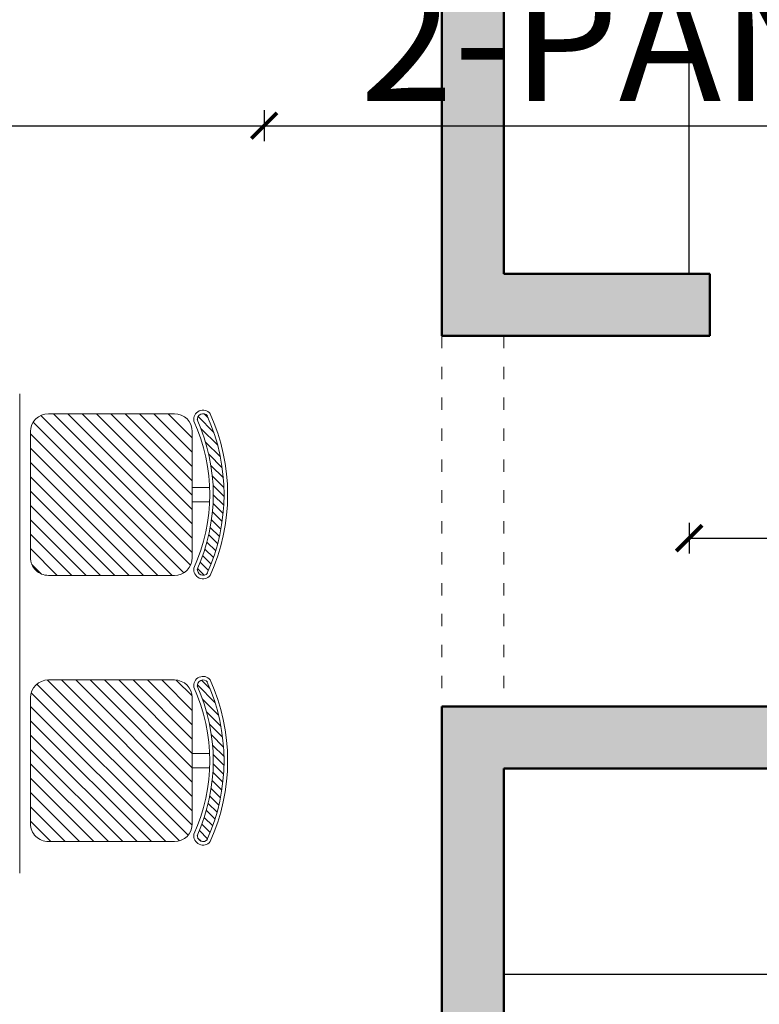
# Model space of a CAD drawing. Units: inches. Extents: x 375 to 1122, y 27 to 1069.
# Tile 149 of 155: x 747 to 819, y 846 to 941. Entities that reach past the tile are written whole.
import ezdxf

# ---------------------------------------------------------------- set-up
doc = ezdxf.new("R2010")
doc.units = ezdxf.units.IN
doc.linetypes.add('ACAD_ISO03W100', pattern=[30, 12, -18])
for name, color, linetype, lineweight in [('A-ANNO-DIMS', 2, 'Continuous', 18), ('A-FLOR-MILL', 55, 'Continuous', 25), ('A-WALL-OVHD', 77, 'ACAD_ISO03W100', 18), ('A-WALL-PATT', 252, 'Continuous', 13), ('Furniture', 30, 'Continuous', 18), ('Walls', 250, 'Continuous', 50)]:
    doc.layers.add(name, color=color, linetype=linetype, lineweight=lineweight)
doc.styles.get("Standard").update_dxf_attribs({"font": 'arial.ttf'})
doc.dimstyles.new('ISO-25', dxfattribs={"dimtxt": 12, "dimasz": 2.5, "dimexe": 1.5, "dimexo": 1.5, "dimtad": 1, "dimdec": 1, "dimlunit": 3, "dimtxsty": 'Standard', "dimblk": 'ARCHTICK', "dimcen": 2.5, "dimadec": 0, "dimazin": 0, "dimtfac": 1, "dimtdec": 1, "dimtmove": 0, "dimatfit": 3, "dimfxl": 1.5, "dimfxlon": 1, "dimarcsym": 0})

# ---------------------------------------------------------------- blocks, each defined once
blk = doc.blocks.new('A$C403C54AD')
at = {"ltscale": 0.05}
for p, q in [((0.9605, 2.0325, -0.0006), (0.9198, 1.9918, -0.0006)), ((0.9888, 2.039, -0.0006), (0.953, 2.0032, -0.0006)), ((1.015, 2.0435, -0.0006), (0.9825, 2.0109, -0.0006)), ((1.0396, 2.0463, -0.0006), (1.0095, 2.0162, -0.0006)), ((1.0628, 2.0477, -0.0006), (1.0346, 2.0195, -0.0006)), ((1.0849, 2.048, -0.0006), (1.0582, 2.0213, -0.0006)), ((1.106, 2.0473, -0.0006), (1.0805, 2.0219, -0.0006)), ((1.1262, 2.0458, -0.0006), (1.1017, 2.0213, -0.0006)), ((1.1456, 2.0435, -0.0006), (1.122, 2.0199, -0.0006)), ((1.1643, 2.0404, -0.0006), (1.1415, 2.0176, -0.0006)), ((1.1824, 2.0368, -0.0006), (1.1603, 2.0146, -0.0006)), ((1.1999, 2.0325, -0.0006), (1.1783, 2.0108, -0.0006)), ((1.6158, 2.0348, -0.0006), (1.5768, 1.9958, -0.0006)), ((1.6434, 2.0406, -0.0006), (1.6087, 2.0059, -0.0006)), ((1.6691, 2.0445, -0.0006), (1.6374, 2.0128, -0.0006)), ((1.6932, 2.0469, -0.0006), (1.6637, 2.0174, -0.0006)), ((1.716, 2.0479, -0.0006), (1.6883, 2.0202, -0.0006)), ((1.7378, 2.0479, -0.0006), (1.7115, 2.0216, -0.0006)), ((1.7586, 2.0469, -0.0006), (1.7335, 2.0218, -0.0006)), ((1.7786, 2.0451, -0.0006), (1.7544, 2.021, -0.0006)), ((1.7978, 2.0426, -0.0006), (1.7744, 2.0193, -0.0006)), ((1.8163, 2.0394, -0.0006), (1.7937, 2.0167, -0.0006)), ((1.8342, 2.0355, -0.0006), (1.8122, 2.0135, -0.0006)), ((0.8939, 2.0094, -0.0006), (0.8844, 1.9999, -0.0006)), ((0.9293, 2.0231, -0.0006), (0.8911, 1.9849, -0.0006)), ((1.2169, 2.0277, -0.0006), (1.1957, 2.0065, -0.0006)), ((1.2333, 2.0223, -0.0006), (1.2126, 2.0016, -0.0006)), ((1.2493, 2.0165, -0.0006), (1.2289, 1.9961, -0.0006)), ((1.2647, 2.0102, -0.0006), (1.2447, 1.9902, -0.0006)), ((1.5517, 2.0142, -0.0006), (1.5308, 1.9933, -0.0006)), ((1.5856, 2.0264, -0.0006), (1.5425, 1.9832, -0.0006)), ((1.8515, 2.0311, -0.0006), (1.8301, 2.0096, -0.0006)), ((1.8683, 2.0261, -0.0006), (1.8473, 2.0051, -0.0006)), ((1.8846, 2.0206, -0.0006), (1.864, 2, -0.0006)), ((1.9004, 2.0146, -0.0006), (1.8801, 1.9943, -0.0006)), ((1.9157, 2.0082, -0.0006), (1.8958, 1.9882, -0.0006)), ((1.2759, 1.9996, -0.0006), (1.26, 1.9837, -0.0006)), ((1.9217, 1.9924, -0.0006), (1.9133, 1.9839, -0.0006)), ((1.2211, 1.9709, -0.0006), (0.8839, 1.6337, -0.0006)), ((1.1862, 1.9709, -0.0006), (0.8839, 1.6685, -0.0006)), ((1.1514, 1.9709, -0.0006), (0.8839, 1.7033, -0.0006)), ((1.1166, 1.9709, -0.0006), (0.8839, 1.7382, -0.0006)), ((1.0818, 1.9709, -0.0006), (0.8839, 1.773, -0.0006)), ((1.0469, 1.9709, -0.0006), (0.8839, 1.8078, -0.0006)), ((1.0121, 1.9709, -0.0006), (0.8839, 1.8427, -0.0006)), ((0.9773, 1.9709, -0.0006), (0.8839, 1.8775, -0.0006)), ((0.9424, 1.9709, -0.0006), (0.8839, 1.9123, -0.0006)), ((1.2517, 1.9667, -0.0006), (0.8881, 1.6031, -0.0006)), ((1.848, 1.9709, -0.0006), (1.5302, 1.6531, -0.0006)), ((1.8131, 1.9709, -0.0006), (1.5302, 1.6879, -0.0006)), ((1.7783, 1.9709, -0.0006), (1.5302, 1.7228, -0.0006)), ((1.7435, 1.9709, -0.0006), (1.5302, 1.7576, -0.0006)), ((1.7087, 1.9709, -0.0006), (1.5302, 1.7924, -0.0006)), ((1.6738, 1.9709, -0.0006), (1.5302, 1.8272, -0.0006)), ((1.639, 1.9709, -0.0006), (1.5302, 1.8621, -0.0006)), ((1.6042, 1.9709, -0.0006), (1.5302, 1.8969, -0.0006)), ((1.8827, 1.9708, -0.0006), (1.5303, 1.6184, -0.0006)), ((1.5691, 1.9706, -0.0006), (1.5304, 1.932, -0.0006)), ((1.9073, 1.9606, -0.0006), (1.5405, 1.5937, -0.0006)), ((1.27, 1.9502, -0.0006), (0.9046, 1.5847, -0.0006)), ((1.9211, 1.9395, -0.0006), (1.5615, 1.58, -0.0006)), ((1.2765, 1.9219, -0.0006), (0.9329, 1.5782, -0.0006)), ((1.9228, 1.9065, -0.0006), (1.5946, 1.5782, -0.0006)), ((1.2765, 1.8871, -0.0006), (0.9677, 1.5782, -0.0006)), ((1.9228, 1.8716, -0.0006), (1.6294, 1.5782, -0.0006)), ((1.2765, 1.8522, -0.0006), (1.0025, 1.5782, -0.0006)), ((1.2765, 1.8174, -0.0006), (1.0374, 1.5782, -0.0006)), ((1.9228, 1.8368, -0.0006), (1.6643, 1.5782, -0.0006)), ((1.9228, 1.802, -0.0006), (1.6991, 1.5782, -0.0006)), ((1.2765, 1.7826, -0.0006), (1.0722, 1.5782, -0.0006)), ((1.2765, 1.7477, -0.0006), (1.107, 1.5782, -0.0006)), ((1.9228, 1.7671, -0.0006), (1.7339, 1.5782, -0.0006)), ((1.9228, 1.7323, -0.0006), (1.7687, 1.5782, -0.0006)), ((1.2765, 1.7129, -0.0006), (1.1418, 1.5782, -0.0006)), ((1.9228, 1.6975, -0.0006), (1.8036, 1.5782, -0.0006)), ((1.2765, 1.6781, -0.0006), (1.1767, 1.5782, -0.0006)), ((1.9228, 1.6627, -0.0006), (1.8384, 1.5782, -0.0006)), ((1.2765, 1.6433, -0.0006), (1.2115, 1.5782, -0.0006)), ((1.9228, 1.6278, -0.0006), (1.8732, 1.5782, -0.0006)), ((1.2732, 1.6051, -0.0006), (1.2497, 1.5816, -0.0006))]:
    blk.add_line(p, q, dxfattribs=at)
for p, q in [((1.0628, 1.9709, -0.0006), (1.0628, 2.0131, -0.0006)), ((1.0977, 1.9709, -0.0006), (1.0977, 2.0131, -0.0006)), ((1.7091, 1.9709, -0.0006), (1.7091, 2.0131, -0.0006)), ((1.744, 1.9709, -0.0006), (1.744, 2.0131, -0.0006)), ((0.9275, 1.9709, -0.0006), (1.2329, 1.9709, -0.0006)), ((1.5738, 1.9709, -0.0006), (1.8792, 1.9709, -0.0006)), ((0.8839, 1.7527, -0.0006), (0.8839, 1.9273, -0.0006)), ((1.2765, 1.9273, -0.0006), (1.2765, 1.6218, -0.0006)), ((1.5302, 1.7527, -0.0006), (1.5302, 1.9273, -0.0006)), ((1.9228, 1.9273, -0.0006), (1.9228, 1.6218, -0.0006)), ((0.8839, 1.6218, -0.0006), (0.8839, 1.7527, -0.0006)), ((1.5302, 1.6218, -0.0006), (1.5302, 1.7527, -0.0006)), ((1.2329, 1.5782, -0.0006), (0.9275, 1.5782, -0.0006)), ((1.8792, 1.5782, -0.0006), (1.5738, 1.5782, -0.0006)), ((0.8357, 1.5519, -0.0006), (1.9992, 1.5519, -0.0006))]:
    blk.add_line(p, q)
for centre, radius, start, end in [((1.0802, 1.5793, -0.0006), 0.4774, 65.7176, 114.2824), ((1.7265, 1.5793, -0.0006), 0.4774, 65.7176, 114.2824), ((1.0802, 1.5793, -0.0006), 0.4687, 65.7176, 114.2824), ((1.7265, 1.5793, -0.0006), 0.4687, 65.7176, 114.2824), ((0.8978, 1.9969, -0.0006), 0.0225, 128.3306, 280.2342), ((1.0802, 1.5793, -0.0006), 0.4425, 65.7176, 114.2824), ((1.0802, 1.5793, -0.0006), 0.4338, 65.7176, 114.2824), ((1.2624, 1.997, -0.0006), 0.0225, 260.3316, 51.1036), ((1.5441, 1.9969, -0.0006), 0.0225, 128.3306, 280.2342), ((1.7265, 1.5793, -0.0006), 0.4425, 65.7176, 114.2824), ((1.7265, 1.5793, -0.0006), 0.4338, 65.7176, 114.2824), ((1.9087, 1.997, -0.0006), 0.0225, 260.3316, 51.1036), ((0.8978, 1.9969, -0.0006), 0.0138, 128.3306, 280.2342), ((1.2624, 1.997, -0.0006), 0.0138, 260.3316, 51.1036), ((1.5441, 1.9969, -0.0006), 0.0138, 128.3306, 280.2342), ((1.9087, 1.997, -0.0006), 0.0138, 260.3316, 51.1036), ((0.9275, 1.9273, -0.0006), 0.0436, 90, 180), ((1.2329, 1.9273, -0.0006), 0.0436, 0, 90), ((1.5738, 1.9273, -0.0006), 0.0436, 90, 180), ((1.8792, 1.9273, -0.0006), 0.0436, 0, 90), ((0.9275, 1.6218, -0.0006), 0.0436, 180, 270), ((1.2329, 1.6218, -0.0006), 0.0436, 270, 0), ((1.5738, 1.6218, -0.0006), 0.0436, 180, 270), ((1.8792, 1.6218, -0.0006), 0.0436, 270, 0)]:
    blk.add_arc(centre, radius, start, end)
blk = doc.blocks.new('KITCHEN-COUNTER-L')
for p, q in [((0, 9), (0, 42)), ((87, 42), (0, 42)), ((87, 0), (87, 42)), ((87, 0), (111, 0))]:
    blk.add_line(p, q)
blk = doc.blocks.new('_ArchTick')
at = {"color": 0, "linetype": 'ByBlock', "const_width": 0.15}
blk.add_lwpolyline([(-0.5, -0.5), (0.5, 0.5)], dxfattribs=at)
blk = doc.blocks.new('*D67')
at = {"layer": 'A-ANNO-DIMS', "color": 0, "lineweight": -2, "transparency": 16777216}
for p, q in [((819.234, 948.294), (819.234, 945.294)), ((853.325, 948.294), (853.325, 945.294)), ((819.234, 946.794), (853.325, 946.794)), ((853.325, 946.794), (1027.891, 946.794))]:
    blk.add_line(p, q, dxfattribs=at)
at = {"layer": 'Defpoints', "color": 0, "transparency": 16777216}
for p in [(819.234, 951.908), (853.325, 951.908), (853.325, 946.794)]:
    blk.add_point(p, dxfattribs=at)
at = {"layer": 'A-ANNO-DIMS', "color": 0, "lineweight": -2, "transparency": 16777216, "xscale": 2.5, "yscale": 2.5, "zscale": 2.5, "rotation": 180}
blk.add_blockref('_ArchTick', (819.234, 946.794), dxfattribs=at)
at = {"layer": 'A-ANNO-DIMS', "color": 0, "lineweight": -2, "transparency": 16777216, "xscale": 2.5, "yscale": 2.5, "zscale": 2.5}
blk.add_blockref('_ArchTick', (853.325, 946.794), dxfattribs=at)
at = {"layer": 'A-ANNO-DIMS', "color": 0, "transparency": 16777216, "insert": (941.858, 953.628), "char_height": 12, "attachment_point": 5}
blk.add_mtext('COOKTOP 2\'-10" TYP.', dxfattribs=at)
blk = doc.blocks.new('*D73')
at = {"layer": 'A-ANNO-DIMS', "color": 0, "lineweight": -2, "transparency": 16777216}
for p, q in [((686.757, 932.428), (686.757, 929.428)), ((770.757, 932.428), (770.757, 929.428)), ((686.757, 930.928), (770.757, 930.928)), ((770.757, 930.928), (987.61, 930.928))]:
    blk.add_line(p, q, dxfattribs=at)
at = {"layer": 'Defpoints', "color": 0, "transparency": 16777216}
for p in [(686.757, 943.528), (770.757, 943.528), (770.757, 930.928)]:
    blk.add_point(p, dxfattribs=at)
at = {"layer": 'A-ANNO-DIMS', "color": 0, "lineweight": -2, "transparency": 16777216, "xscale": 2.5, "yscale": 2.5, "zscale": 2.5, "rotation": 180}
blk.add_blockref('_ArchTick', (686.757, 930.928), dxfattribs=at)
at = {"layer": 'A-ANNO-DIMS', "color": 0, "lineweight": -2, "transparency": 16777216, "xscale": 2.5, "yscale": 2.5, "zscale": 2.5}
blk.add_blockref('_ArchTick', (770.757, 930.928), dxfattribs=at)
at = {"layer": 'A-ANNO-DIMS', "color": 0, "transparency": 16777216, "insert": (880.433, 937.757), "char_height": 12, "attachment_point": 5}
blk.add_mtext('2-PANEL SLIDER 7\'-0" TYP.', dxfattribs=at)
blk = doc.blocks.new('*D77')
at = {"layer": 'A-ANNO-DIMS', "color": 0, "lineweight": -2, "transparency": 16777216}
for p, q in [((812.007, 892.378), (812.007, 889.378)), ((923.007, 892.378), (923.007, 889.378)), ((812.007, 890.878), (923.007, 890.878)), ((923.007, 890.878), (1101.821, 890.878))]:
    blk.add_line(p, q, dxfattribs=at)
at = {"layer": 'Defpoints', "color": 0, "transparency": 16777216}
for p in [(812.007, 907.528), (923.007, 907.528), (923.007, 890.878)]:
    blk.add_point(p, dxfattribs=at)
at = {"layer": 'A-ANNO-DIMS', "color": 0, "lineweight": -2, "transparency": 16777216, "xscale": 2.5, "yscale": 2.5, "zscale": 2.5, "rotation": 180}
blk.add_blockref('_ArchTick', (812.007, 890.878), dxfattribs=at)
at = {"layer": 'A-ANNO-DIMS', "color": 0, "lineweight": -2, "transparency": 16777216, "xscale": 2.5, "yscale": 2.5, "zscale": 2.5}
blk.add_blockref('_ArchTick', (923.007, 890.878), dxfattribs=at)
at = {"layer": 'A-ANNO-DIMS', "color": 0, "transparency": 16777216, "insert": (1013.664, 897.716), "char_height": 12, "attachment_point": 5}
blk.add_mtext('L-COUNTER 9\'-3" TYP.', dxfattribs=at)
blk = doc.blocks.new('*D85')
at = {"layer": 'A-ANNO-DIMS', "color": 0, "lineweight": -2, "transparency": 16777216}
for p, q in [((401.507, 868.528), (398.507, 868.528)), ((400.007, 814.528), (400.007, 868.528)), ((401.507, 814.528), (398.507, 814.528))]:
    blk.add_line(p, q, dxfattribs=at)
at = {"layer": 'Defpoints', "color": 0, "transparency": 16777216}
for p in [(400.007, 868.528), (845.007, 868.528), (845.007, 814.528)]:
    blk.add_point(p, dxfattribs=at)
at = {"layer": 'A-ANNO-DIMS', "color": 0, "lineweight": -2, "transparency": 16777216, "xscale": 2.5, "yscale": 2.5, "zscale": 2.5}
for p, rotation in [((400.007, 868.528), 90), ((400.007, 814.528), 270)]:
    blk.add_blockref('_ArchTick', p, dxfattribs=dict(at, rotation=rotation))
at = {"layer": 'A-ANNO-DIMS', "color": 0, "transparency": 16777216, "insert": (393.255, 841.528), "char_height": 12, "attachment_point": 5, "rotation": 90}
blk.add_mtext('4\'-6"', dxfattribs=at)
blk = doc.blocks.new('*D88')
at = {"layer": 'A-ANNO-DIMS', "color": 0, "lineweight": -2, "transparency": 16777216}
for p, q in [((731.007, 1052.528), (731.007, 1055.528)), ((854.007, 1052.528), (854.007, 1055.528)), ((731.007, 1054.028), (854.007, 1054.028))]:
    blk.add_line(p, q, dxfattribs=at)
at = {"layer": 'Defpoints', "color": 0, "transparency": 16777216}
for p in [(854.007, 1054.028), (731.007, 502.528), (854.007, 502.528)]:
    blk.add_point(p, dxfattribs=at)
at = {"layer": 'A-ANNO-DIMS', "color": 0, "lineweight": -2, "transparency": 16777216, "xscale": 2.5, "yscale": 2.5, "zscale": 2.5, "rotation": 180}
blk.add_blockref('_ArchTick', (731.007, 1054.028), dxfattribs=at)
at = {"layer": 'A-ANNO-DIMS', "color": 0, "lineweight": -2, "transparency": 16777216, "xscale": 2.5, "yscale": 2.5, "zscale": 2.5}
blk.add_blockref('_ArchTick', (854.007, 1054.028), dxfattribs=at)
at = {"layer": 'A-ANNO-DIMS', "color": 0, "transparency": 16777216, "insert": (792.507, 1060.784), "char_height": 12, "attachment_point": 5}
blk.add_mtext('10\'-3"', dxfattribs=at)
blk = doc.blocks.new('*D91')
at = {"layer": 'A-ANNO-DIMS', "color": 0, "lineweight": -2, "transparency": 16777216}
for p, q in [((728.007, 1052.528), (728.007, 1055.528)), ((788.007, 1052.528), (788.007, 1055.528)), ((728.007, 1054.028), (788.007, 1054.028))]:
    blk.add_line(p, q, dxfattribs=at)
at = {"layer": 'Defpoints', "color": 0, "transparency": 16777216}
for p in [(788.007, 1054.028), (728.007, 774.028), (788.007, 774.028)]:
    blk.add_point(p, dxfattribs=at)
at = {"layer": 'A-ANNO-DIMS', "color": 0, "lineweight": -2, "transparency": 16777216, "xscale": 2.5, "yscale": 2.5, "zscale": 2.5, "rotation": 180}
blk.add_blockref('_ArchTick', (728.007, 1054.028), dxfattribs=at)
at = {"layer": 'A-ANNO-DIMS', "color": 0, "lineweight": -2, "transparency": 16777216, "xscale": 2.5, "yscale": 2.5, "zscale": 2.5}
blk.add_blockref('_ArchTick', (788.007, 1054.028), dxfattribs=at)
at = {"layer": 'A-ANNO-DIMS', "color": 0, "transparency": 16777216, "insert": (758.007, 1060.78), "char_height": 12, "attachment_point": 5}
blk.add_mtext('5\'-0"', dxfattribs=at)

msp = doc.modelspace()

# ---------------------------------------------------------------- hatches: boundary and pattern name
at = {"layer": 'A-WALL-PATT'}
h = msp.add_hatch(color=256, dxfattribs=at)
h.dxf.hatch_style = 1
h.paths.add_polyline_path([(962.007, 388.528), (989.007, 388.528), (989.007, 394.528), (962.007, 394.528), (932.007, 394.528), (932.007, 397.528), (923.007, 397.528), (923.007, 394.528), (842.007, 394.528), (842.007, 334.528), (839.507, 334.528), (839.507, 328.528), (854.007, 328.528), (854.007, 334.528), (848.007, 334.528), (848.007, 388.528), (953.007, 388.528), (953.007, 356.081), (962.007, 356.081), (962.007, 358.554), (989.007, 358.554), (989.007, 364.554), (962.007, 364.554)])
h.paths.add_polyline_path([(989.007, 502.528), (932.007, 502.528), (932.007, 583.528), (932.007, 593.528), (923.007, 593.528), (923.007, 583.528), (854.007, 583.528), (854.007, 556.528), (863.007, 556.528), (863.007, 574.528), (923.007, 574.528), (923.007, 502.528), (863.007, 502.528), (863.007, 520.528), (854.007, 520.528), (854.007, 502.528), (773.007, 502.528), (773.007, 493.528), (788.007, 493.528), (788.007, 402.028), (722.007, 402.028), (722.007, 373.528), (728.007, 373.528), (728.007, 396.028), (788.007, 396.028), (788.007, 373.528), (794.007, 373.528), (794.007, 430.528), (814.007, 430.528), (814.007, 436.528), (794.007, 436.528), (794.007, 493.528), (923.007, 493.528), (923.007, 487.528), (932.007, 487.528), (932.007, 493.528), (983.007, 493.528), (983.007, 473.528), (989.007, 473.528)])
h.paths.add_polyline_path([(797.007, 325.528), (805.007, 325.528), (805.007, 328.528), (807.507, 328.528), (807.507, 334.528), (791.007, 334.528), (791.007, 226.528), (770.757, 226.528), (770.757, 217.528), (791.007, 217.528), (791.007, 187.528), (855.007, 187.528), (855.007, 196.528), (797.007, 196.528)])
h.paths.add_polyline_path([(989.007, 238.528), (962.007, 238.528), (962.007, 256.424), (953.007, 256.424), (953.007, 229.528), (980.007, 229.528), (980.007, 196.528), (915.007, 196.528), (915.007, 187.528), (989.007, 187.528)])
h.paths.add_polyline_path([(962.007, 334.528), (884.007, 334.528), (884.007, 328.528), (918.007, 328.528), (918.007, 325.528), (932.007, 325.528), (932.007, 328.528), (953.007, 328.528), (953.007, 304.424), (962.007, 304.424)])
h.paths.add_polyline_path([(606.507, 283.528), (609.507, 283.528), (609.507, 289.528), (600.507, 289.528), (600.507, 196.528), (578.507, 196.528), (578.507, 187.528), (606.507, 187.528), (606.507, 196.528)])
h.paths.add_polyline_path([(666.507, 292.528), (660.507, 292.528), (660.507, 289.528), (633.507, 289.528), (633.507, 283.528), (660.507, 283.528), (660.507, 196.528), (628.007, 196.528), (628.007, 187.528), (630.534, 187.528), (630.534, 160.528), (636.534, 160.528), (636.534, 187.528), (660.507, 187.528), (660.507, 160.528), (666.507, 160.528), (666.507, 217.528), (686.757, 217.528), (686.757, 226.528), (666.507, 226.528)])
h.paths.add_polyline_path([(480.507, 256.424), (471.507, 256.424), (471.507, 238.528), (444.507, 238.528), (444.507, 187.528), (518.507, 187.528), (518.507, 196.528), (453.507, 196.528), (453.507, 229.528), (480.507, 229.528)])
h.paths.add_polyline_path([(480.507, 328.528), (652.507, 328.528), (652.507, 325.528), (660.507, 325.528), (660.507, 322.528), (666.507, 322.528), (666.507, 334.528), (507.507, 334.528), (507.507, 360.528), (498.507, 360.528), (498.507, 334.528), (471.507, 334.528), (471.507, 304.424), (480.507, 304.424)])
h.paths.add_polyline_path([(507.507, 484.528), (498.507, 484.528), (498.507, 444.528), (507.507, 444.528), (507.507, 454.528), (621.507, 454.528), (621.507, 460.528), (507.507, 460.528)])
h.paths.add_polyline_path([(672.507, 604.528), (683.257, 604.528), (683.257, 613.528), (669.507, 613.528), (669.507, 649.528), (663.507, 649.528), (663.507, 589.528), (507.507, 589.528), (507.507, 613.528), (498.507, 613.528), (498.507, 556.528), (507.507, 556.528), (507.507, 580.528), (663.507, 580.528), (663.507, 520.528), (669.507, 520.528), (669.507, 556.528), (683.257, 556.528), (683.257, 565.528), (672.507, 565.528)])
h.paths.add_polyline_path([(731.007, 667.528), (734.007, 667.528), (734.007, 676.528), (728.007, 676.528), (728.007, 715.528), (657.507, 715.528), (657.507, 709.528), (663.507, 709.528), (663.507, 673.528), (669.507, 673.528), (669.507, 709.528), (722.007, 709.528), (722.007, 613.528), (704.757, 613.528), (704.757, 604.528), (722.007, 604.528), (722.007, 565.528), (704.757, 565.528), (704.757, 556.528), (722.007, 556.528), (722.007, 502.528), (722.007, 460.528), (669.507, 460.528), (669.507, 496.528), (663.507, 496.528), (663.507, 460.528), (657.507, 460.528), (657.507, 454.528), (728.007, 454.528), (728.007, 493.528), (734.007, 493.528), (734.007, 502.528), (731.007, 502.528)])
h.paths.add_polyline_path([(986.007, 718.528), (959.007, 718.528), (959.007, 727.528), (950.007, 727.528), (950.007, 709.528), (977.007, 709.528), (977.007, 676.528), (794.007, 676.528), (794.007, 805.528), (802.007, 805.528), (802.007, 808.528), (804.507, 808.528), (804.507, 814.528), (788.007, 814.528), (788.007, 774.028), (728.007, 774.028), (728.007, 796.528), (722.007, 796.528), (722.007, 768.028), (788.007, 768.028), (788.007, 676.528), (773.007, 676.528), (773.007, 667.528), (923.007, 667.528), (923.007, 657.528), (932.007, 657.528), (932.007, 667.528), (986.007, 667.528)])
h.paths.add_polyline_path([(621.507, 715.528), (507.507, 715.528), (507.507, 733.528), (498.507, 733.528), (498.507, 715.528), (498.507, 685.528), (507.507, 685.528), (507.507, 709.528), (621.507, 709.528)])
h.paths.add_polyline_path([(666.507, 847.028), (660.507, 847.028), (660.507, 844.528), (652.507, 844.528), (652.507, 841.528), (480.507, 841.528), (480.507, 859.528), (471.507, 859.528), (471.507, 835.528), (498.507, 835.528), (498.507, 817.528), (507.507, 817.528), (507.507, 835.528), (666.507, 835.528)])
h.paths.add_polyline_path([(480.507, 940.528), (453.507, 940.528), (453.507, 973.528), (518.507, 973.528), (518.507, 982.528), (444.507, 982.528), (444.507, 931.528), (471.507, 931.528), (471.507, 907.528), (480.507, 907.528)])
h.paths.add_polyline_path([(606.507, 982.528), (578.507, 982.528), (578.507, 973.528), (600.507, 973.528), (600.507, 880.528), (609.507, 880.528), (609.507, 886.528), (606.507, 886.528)])
h.paths.add_polyline_path([(666.507, 943.528), (686.757, 943.528), (686.757, 952.528), (666.507, 952.528), (666.507, 1009.528), (660.507, 1009.528), (660.507, 982.528), (636.534, 982.528), (636.534, 1009.528), (630.534, 1009.528), (630.534, 982.528), (628.007, 982.528), (628.007, 973.528), (660.507, 973.528), (660.507, 886.528), (633.507, 886.528), (633.507, 880.528), (660.507, 880.528), (660.507, 877.028), (666.507, 877.028)])
h.paths.add_polyline_path([(986.007, 874.528), (932.007, 874.528), (932.007, 877.528), (923.007, 877.528), (923.007, 874.528), (788.007, 874.528), (788.007, 868.528), (788.007, 844.528), (794.007, 844.528), (794.007, 868.528), (839.007, 868.528), (839.007, 814.528), (836.507, 814.528), (836.507, 808.528), (851.007, 808.528), (851.007, 814.528), (845.007, 814.528), (845.007, 868.528), (986.007, 868.528)])
h.paths.add_polyline_path([(959.007, 838.554), (986.007, 838.554), (986.007, 844.554), (959.007, 844.554), (959.007, 847.028), (950.007, 847.028), (950.007, 814.528), (881.007, 814.528), (881.007, 808.528), (918.007, 808.528), (918.007, 805.528), (932.007, 805.528), (932.007, 808.528), (950.007, 808.528), (950.007, 793.528), (959.007, 793.528)])
h.paths.add_polyline_path([(986.007, 982.528), (899.007, 982.528), (899.007, 973.528), (923.007, 973.528), (923.007, 967.528), (932.007, 967.528), (932.007, 973.528), (980.007, 973.528), (980.007, 953.528), (986.007, 953.528)])
h.paths.add_polyline_path([(851.007, 982.528), (788.007, 982.528), (788.007, 952.528), (770.757, 952.528), (770.757, 943.528), (788.007, 943.528), (788.007, 910.528), (814.007, 910.528), (814.007, 916.528), (794.007, 916.528), (794.007, 973.528), (851.007, 973.528)])

# ---------------------------------------------------------------- linework, layer by layer
at = {"layer": 'A-FLOR-MILL'}
msp.add_line((839.007, 848.528), (794.007, 848.528), dxfattribs=at)
at = {"layer": 'A-WALL-OVHD', "ltscale": 0.1}
for p, q in [((788.007, 910.528), (788.007, 874.528)), ((794.007, 910.528), (794.007, 874.528))]:
    msp.add_line(p, q, dxfattribs=at)
at = {"layer": 'Walls'}
for p, q in [((794.007, 916.528), (794.007, 973.528)), ((788.007, 910.528), (788.007, 943.528)), ((814.007, 916.528), (794.007, 916.528)), ((814.007, 910.528), (814.007, 916.528)), ((814.007, 910.528), (788.007, 910.528)), ((788.007, 868.528), (788.007, 874.528)), ((923.007, 874.528), (788.007, 874.528)), ((788.007, 868.528), (788.007, 844.528)), ((794.007, 844.528), (794.007, 868.528)), ((839.007, 868.528), (794.007, 868.528))]:
    msp.add_line(p, q, dxfattribs=at)

# ---------------------------------------------------------------- block references
at = {"layer": 'A-FLOR-MILL'}
msp.add_blockref('KITCHEN-COUNTER-L', (812.007, 907.528), dxfattribs=at)
at = {"layer": 'Furniture', "xscale": 39.9918517141215, "yscale": 39.9918517141215, "zscale": 39.9918517141215, "rotation": 270}
msp.add_blockref('A$C403C54AD', (684.955, 938.316, 0.024), dxfattribs=at)

# ---------------------------------------------------------------- dimensions: what is measured, and where the dimension line sits
at = {"layer": 'A-ANNO-DIMS'}
for base, p1, p2, picture, middle in [((788.007, 1054.028), (728.007, 774.028), (788.007, 774.028), '*D91', (758.007, 1060.78)), ((854.007, 1054.028), (731.007, 502.528), (854.007, 502.528), '*D88', (792.507, 1060.784))]:
    dim = msp.add_linear_dim(base=base, p1=p1, p2=p2, dimstyle='ISO-25', override={"dimdec": 1, "dimlfac": 1, "dimrnd": 0, "dimzin": 1, "dimdsep": 46, "dimlunit": 4, "dimfrac": 2}, dxfattribs=at)
    dim.commit()
    dim.dimension.update_dxf_attribs({"geometry": picture, "text_midpoint": middle})
for base, p1, p2, text, picture, middle in [((853.325, 946.794), (819.234, 951.908), (853.325, 951.908), 'COOKTOP <> TYP.', '*D67', (941.858, 953.628)), ((770.757, 930.928), (686.757, 943.528), (770.757, 943.528), '2-PANEL SLIDER <> TYP.', '*D73', (880.433, 937.757)), ((923.007, 890.878), (812.007, 907.528), (923.007, 907.528), 'L-COUNTER <> TYP.', '*D77', (1013.664, 897.716))]:
    dim = msp.add_linear_dim(base=base, p1=p1, p2=p2, text=text, dimstyle='ISO-25', override={"dimdec": 1, "dimlfac": 1, "dimrnd": 0, "dimzin": 1, "dimdsep": 46, "dimlunit": 4, "dimfrac": 2}, dxfattribs=at)
    dim.commit()
    dim.dimension.update_dxf_attribs({"geometry": picture, "text_midpoint": middle})
dim = msp.add_linear_dim(base=(400.007, 868.528), p1=(845.007, 814.528), p2=(845.007, 868.528), angle=90, dimstyle='ISO-25', override={"dimdec": 1, "dimlfac": 1, "dimrnd": 0, "dimzin": 1, "dimdsep": 46, "dimlunit": 4, "dimfrac": 2}, dxfattribs=at)
dim.commit()
dim.dimension.update_dxf_attribs({"geometry": '*D85', "text_midpoint": (393.255, 841.528)})

doc.saveas('drawing.dxf')
